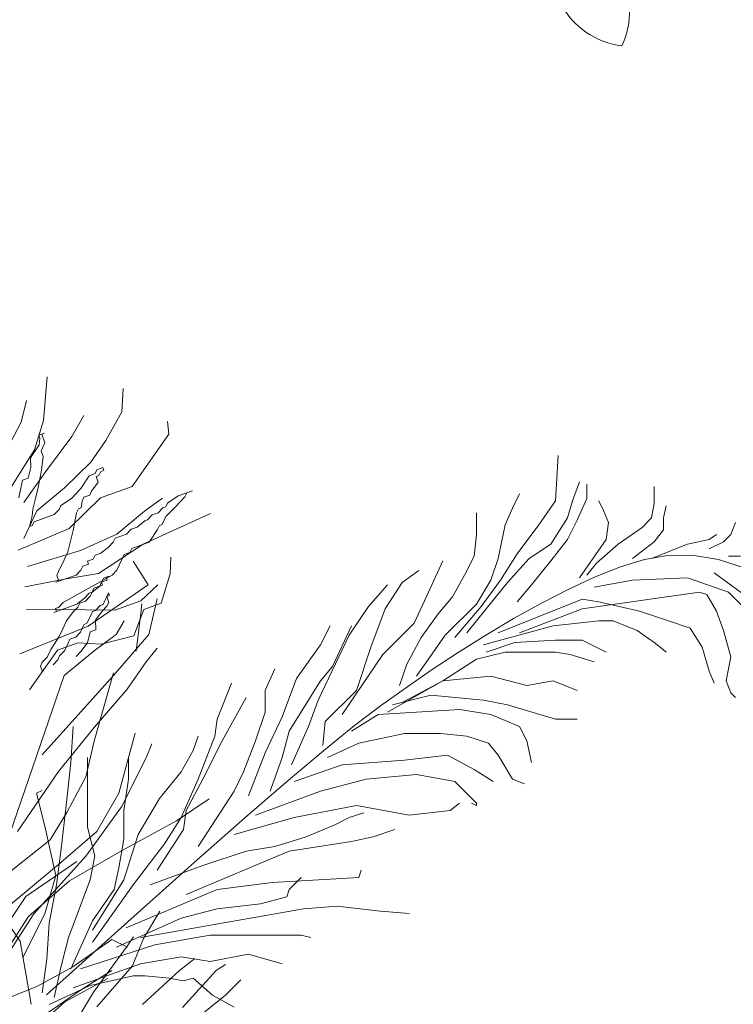
# Model space of a CAD drawing. Units: millimetres. Extents: x 595116 to 630915, y 909473 to 920225.
# Tile 74 of 134: x 629629.81 to 629636.468, y 919276.713 to 919285.898. Entities that reach past the tile are written whole.
import ezdxf

# ---------------------------------------------------------------- set-up
doc = ezdxf.new("R2010")
doc.units = ezdxf.units.MM
doc.layers.add('Dimension', color=3, linetype='Continuous', lineweight=18)
doc.layers.add('L-PLNT', color=85, linetype='Continuous', lineweight=13)
doc.styles.get("Standard").update_dxf_attribs({"font": 'arial.ttf'})
doc.dimstyles.new('ISO-25', dxfattribs={"dimtxt": 9, "dimasz": 6, "dimexe": 1.25, "dimexo": 0.625, "dimtad": 1, "dimlunit": 4, "dimtxsty": 'Standard', "dimcen": 2.5, "dimadec": 0, "dimazin": 0, "dimtfac": 1, "dimtmove": 0, "dimatfit": 3, "dimfxl": 1, "dimarcsym": 0})

# ---------------------------------------------------------------- blocks, each defined once
blk = doc.blocks.new('A$C4FB75ABC')
for p, q in [((2.8876, 3.7608), (2.897, 3.8696)), ((3.0823, 3.7823), (3.0858, 3.8403)), ((2.8322, 3.7571), (2.8454, 3.8105)), ((2.9584, 3.7215), (2.9885, 3.7729)), ((3.043, 3.7114), (3.0823, 3.7823)), ((2.7745, 3.6472), (2.8322, 3.7571)), ((2.8652, 3.6879), (2.8876, 3.7608)), ((3.1994, 3.7272), (3.1962, 3.7584)), ((2.8907, 3.7295), (2.8764, 3.7244)), ((2.8764, 3.7244), (2.8789, 3.7172)), ((2.8835, 3.727), (2.8907, 3.7295)), ((2.8913, 3.7054), (2.8835, 3.727)), ((2.893, 3.6331), (2.9584, 3.7215)), ((3.1085, 3.5972), (3.1994, 3.7272)), ((2.8769, 3.7003), (2.856, 3.6684)), ((2.8789, 3.7172), (2.8769, 3.7003)), ((2.8821, 3.6859), (2.8913, 3.7054)), ((3.0058, 3.6575), (3.043, 3.7114)), ((2.7932, 3.5729), (2.8652, 3.6879)), ((2.8873, 3.6716), (2.8821, 3.6859)), ((2.8833, 3.6377), (2.8873, 3.6716)), ((4.1608, 3.5609), (4.1668, 3.6742)), ((2.856, 3.6684), (2.8566, 3.6443)), ((2.9398, 3.5932), (3.0058, 3.6575)), ((2.8394, 3.5571), (2.893, 3.6331)), ((2.8566, 3.6443), (2.85, 3.6176)), ((2.8746, 3.5941), (2.8833, 3.6377)), ((3.0017, 3.6236), (2.9808, 3.5918)), ((3.0161, 3.6288), (3.0017, 3.6236)), ((3.0207, 3.6385), (3.0161, 3.6288)), ((3.0187, 3.6216), (3.0258, 3.6242)), ((3.035, 3.6437), (3.0207, 3.6385)), ((3.0258, 3.6242), (3.0304, 3.6339)), ((3.0304, 3.6339), (3.0376, 3.6365)), ((3.0376, 3.6365), (3.035, 3.6437)), ((2.8356, 3.6125), (2.827, 3.5688)), ((2.85, 3.6176), (2.8356, 3.6125)), ((3.0075, 3.5852), (3.0238, 3.6072)), ((3.0238, 3.6072), (3.0187, 3.6216)), ((4.2026, 3.5609), (4.2205, 3.6086)), ((4.2384, 3.5668), (4.2384, 3.6026)), ((2.868, 3.5674), (2.8746, 3.5941)), ((2.8712, 3.5361), (2.9398, 3.5932)), ((2.969, 3.5794), (2.9573, 3.5671)), ((2.9808, 3.5918), (2.969, 3.5794)), ((2.9885, 3.5702), (3.0029, 3.5754)), ((3.0029, 3.5754), (3.0075, 3.5852)), ((3.0296, 3.5688), (3.1085, 3.5972)), ((3.2224, 3.5733), (3.1962, 3.5558)), ((3.2582, 3.5862), (3.2224, 3.5733)), ((3.2393, 3.5713), (3.2439, 3.5811)), ((3.2439, 3.5811), (3.2582, 3.5862)), ((4.0535, 3.543), (4.0714, 3.5788)), ((4.4054, 3.5549), (4.4054, 3.5967)), ((2.8614, 3.5407), (2.868, 3.5674)), ((2.9312, 3.5496), (2.9266, 3.5398)), ((2.9573, 3.5671), (2.9312, 3.5496)), ((2.9518, 3.4922), (3.0296, 3.5688)), ((2.9819, 3.5435), (2.984, 3.5605)), ((2.984, 3.5605), (2.9885, 3.5702)), ((3.1389, 3.5352), (3.1839, 3.5676)), ((3.1962, 3.5558), (3.1917, 3.5461)), ((3.2158, 3.5466), (3.2393, 3.5713)), ((4.1191, 3.5013), (4.1608, 3.5609)), ((4.1907, 3.5192), (4.2026, 3.5609)), ((4.2145, 3.5132), (4.2384, 3.5668)), ((4.2801, 3.537), (4.2682, 3.5609)), ((4.3994, 3.5192), (4.4054, 3.5549)), ((4.4293, 3.5192), (4.4352, 3.549)), ((2.8391, 3.4678), (2.8712, 3.5361)), ((2.8594, 3.5238), (2.8614, 3.5407)), ((2.9148, 3.5275), (2.8646, 3.5094)), ((2.9266, 3.5398), (2.9148, 3.5275)), ((2.9616, 3.4876), (2.9702, 3.5312)), ((2.9702, 3.5312), (2.9748, 3.541)), ((2.9748, 3.541), (2.9819, 3.5435)), ((3.0703, 3.4781), (3.1389, 3.5352)), ((3.136, 3.4531), (3.303, 3.5294)), ((3.1584, 3.526), (3.1466, 3.5136)), ((3.1727, 3.5311), (3.1584, 3.526)), ((3.1845, 3.5435), (3.1727, 3.5311)), ((3.1917, 3.5461), (3.1845, 3.5435)), ((3.1922, 3.522), (3.2158, 3.5466)), ((3.964, 3.4774), (3.964, 3.5311)), ((4.0356, 3.5013), (4.0535, 3.543)), ((4.2921, 3.5072), (4.2801, 3.537)), ((2.8528, 3.4971), (2.8594, 3.5238)), ((2.8646, 3.5094), (2.86, 3.4997)), ((3.1394, 3.5111), (3.1205, 3.4961)), ((3.1466, 3.5136), (3.1394, 3.5111)), ((3.1713, 3.4901), (3.1759, 3.4999)), ((3.1759, 3.4999), (3.1831, 3.5024)), ((3.1831, 3.5024), (3.1922, 3.522)), ((4.0177, 3.4178), (4.0356, 3.5013)), ((4.0654, 3.4297), (4.1191, 3.5013)), ((4.1489, 3.4536), (4.1907, 3.5192)), ((4.1907, 3.4655), (4.2145, 3.5132)), ((4.2861, 3.4655), (4.2921, 3.5072)), ((4.3756, 3.4953), (4.3994, 3.5192)), ((4.4293, 3.4893), (4.4293, 3.5192)), ((4.5963, 3.4774), (4.6082, 3.5072)), ((2.8253, 3.4385), (2.9518, 3.4922)), ((2.86, 3.4997), (2.8528, 3.4971)), ((2.9484, 3.4342), (2.9616, 3.4876)), ((2.9797, 3.4374), (3.0703, 3.4781)), ((3.0944, 3.4786), (3.0657, 3.4683)), ((3.1062, 3.491), (3.0944, 3.4786)), ((3.1205, 3.4961), (3.1062, 3.491)), ((3.1503, 3.4583), (3.1713, 3.4901)), ((3.958, 3.4238), (3.964, 3.4774)), ((4.3159, 3.4536), (4.3756, 3.4953)), ((4.4054, 3.4595), (4.4293, 3.4893)), ((4.5426, 3.4655), (4.5605, 3.4774)), ((4.5784, 3.4595), (4.5963, 3.4774)), ((3.0244, 3.3805), (3.136, 3.4531)), ((3.0611, 3.4586), (3.0494, 3.4462)), ((3.0657, 3.4683), (3.0611, 3.4586)), ((3.1073, 3.4428), (3.1503, 3.4583)), ((4.0952, 3.4178), (4.1489, 3.4536)), ((4.1489, 3.4118), (4.1907, 3.4655)), ((4.2205, 3.3701), (4.2861, 3.4655)), ((4.2622, 3.4059), (4.3159, 3.4536)), ((4.3517, 3.4178), (4.4054, 3.4595)), ((4.3994, 3.4178), (4.4889, 3.4536)), ((4.4889, 3.4536), (4.5426, 3.4655)), ((4.5426, 3.4416), (4.5784, 3.4595)), ((2.848, 3.3981), (2.9797, 3.4374)), ((2.9392, 3.4147), (2.9484, 3.4342)), ((3.0304, 3.4313), (3.0161, 3.4262)), ((3.0494, 3.4462), (3.0304, 3.4313)), ((3.07, 3.3888), (3.0884, 3.4279)), ((3.0884, 3.4279), (3.1027, 3.433)), ((3.1027, 3.433), (3.1073, 3.4428)), ((4.0237, 3.3641), (4.0654, 3.4297)), ((2.9254, 3.3854), (2.9392, 3.4147)), ((2.9997, 3.4041), (2.9854, 3.3989)), ((3.0115, 3.4164), (2.9972, 3.4112)), ((2.9972, 3.4112), (2.9997, 3.4041)), ((3.0161, 3.4262), (3.0115, 3.4164)), ((3.1481, 3.3521), (3.1105, 3.4115)), ((3.2028, 3.3799), (3.2043, 3.4209)), ((3.8447, 3.3343), (3.8805, 3.4118)), ((3.9342, 3.3761), (3.958, 3.4238)), ((3.9998, 3.3641), (4.0177, 3.4178)), ((4.0415, 3.3582), (4.0952, 3.4178)), ((4.1012, 3.3522), (4.1489, 3.4118)), ((4.2384, 3.3761), (4.2622, 3.4059)), ((4.322, 3.3969), (4.3813, 3.4152)), ((4.3813, 3.4152), (4.4396, 3.4254)), ((4.4396, 3.4254), (4.5001, 3.426)), ((4.5001, 3.426), (4.5657, 3.4153)), ((4.5657, 3.4153), (4.6395, 3.3917)), ((4.5903, 3.4238), (4.6201, 3.4238)), ((2.9208, 3.3757), (2.9254, 3.3854)), ((2.9403, 3.3665), (3.0244, 3.3805)), ((2.9808, 3.3891), (2.969, 3.3768)), ((2.9854, 3.3989), (2.9808, 3.3891)), ((3.0583, 3.3765), (3.07, 3.3888)), ((3.1805, 3.307), (3.2028, 3.3799)), ((3.7791, 3.3582), (3.8208, 3.388)), ((4.2593, 3.3722), (4.322, 3.3969)), ((4.5545, 3.382), (4.6858, 3.2866)), ((2.8419, 3.3473), (2.9403, 3.3665)), ((2.969, 3.3768), (2.9188, 3.3587)), ((2.9188, 3.3587), (2.926, 3.3613)), ((2.926, 3.3613), (2.9208, 3.3757)), ((2.9369, 3.3085), (3.0583, 3.3765)), ((3.0322, 3.359), (3.0276, 3.3492)), ((3.0367, 3.3687), (3.0322, 3.359)), ((3.0322, 3.359), (3.0465, 3.3642)), ((3.0347, 3.3518), (3.0322, 3.359)), ((3.0511, 3.3739), (3.0367, 3.3687)), ((3.0439, 3.3713), (3.0511, 3.3739)), ((3.0465, 3.3642), (3.0439, 3.3713)), ((3.7373, 3.2926), (3.7791, 3.3582)), ((3.9044, 3.3224), (3.9342, 3.3761)), ((3.964, 3.3045), (3.9998, 3.3641)), ((3.9759, 3.2986), (4.0237, 3.3641)), ((3.9879, 3.2926), (4.0415, 3.3582)), ((4.1935, 3.342), (4.2593, 3.3722)), ((4.2563, 3.3463), (4.3517, 3.3641)), ((4.3517, 3.3641), (4.4889, 3.3701)), ((4.4889, 3.3701), (4.5903, 3.3343)), ((3.0015, 3.3317), (2.9897, 3.3194)), ((2.9986, 3.2497), (3.1481, 3.3521)), ((3.0086, 3.3343), (3.0015, 3.3317)), ((3.004, 3.3246), (3.0086, 3.3343)), ((3.0276, 3.3492), (3.0086, 3.3343)), ((3.0086, 3.3343), (3.0132, 3.3441)), ((3.0132, 3.3441), (3.0347, 3.3518)), ((3.0497, 3.3329), (3.0451, 3.3231)), ((3.0522, 3.3257), (3.0497, 3.3329)), ((3.1297, 3.313), (3.1722, 3.3526)), ((3.6956, 3.2986), (3.7433, 3.3522)), ((3.8089, 3.2568), (3.8447, 3.3343)), ((4.0654, 3.3105), (4.1012, 3.3522)), ((4.1256, 3.3072), (4.1935, 3.342)), ((4.2265, 3.2926), (4.5187, 3.3343)), ((4.5187, 3.3343), (4.5366, 3.3284)), ((4.5903, 3.3343), (4.644, 3.2807)), ((2.9708, 3.3045), (2.9134, 3.2838)), ((2.9251, 3.2962), (2.9369, 3.3085)), ((2.9897, 3.3194), (2.9708, 3.3045)), ((2.9733, 3.2973), (2.9779, 3.3071)), ((2.9779, 3.3071), (2.9923, 3.3122)), ((2.9923, 3.3122), (3.004, 3.3246)), ((3.0359, 3.3036), (3.0405, 3.3134)), ((3.0405, 3.3134), (3.0451, 3.3231)), ((3.0451, 3.3231), (3.0522, 3.3257)), ((3.0451, 3.3231), (3.0502, 3.3088)), ((3.0502, 3.3088), (3.0456, 3.299)), ((3.0651, 3.2898), (3.1297, 3.313)), ((3.1303, 3.2889), (3.1323, 3.3059)), ((3.1374, 3.2915), (3.1805, 3.307)), ((3.1501, 3.2292), (3.1706, 3.3178)), ((3.8686, 3.2807), (3.9044, 3.3224)), ((3.8865, 3.227), (3.964, 3.3045)), ((4.0177, 3.233), (4.2265, 3.3164)), ((4.0565, 3.2687), (4.1256, 3.3072)), ((4.2265, 3.3164), (4.2682, 3.3105)), ((4.2682, 3.3105), (4.3696, 3.2866)), ((4.5366, 3.3284), (4.5605, 3.2866)), ((2.8457, 3.2919), (3.0651, 3.2898)), ((2.9134, 3.2838), (2.9206, 3.2864)), ((2.918, 3.2936), (2.9251, 3.2962)), ((2.9206, 3.2864), (2.918, 3.2936)), ((2.9452, 3.2629), (2.9616, 3.285)), ((2.9616, 3.285), (2.9733, 3.2973)), ((3.0052, 3.2763), (3.0098, 3.2861)), ((3.0098, 3.2861), (3.0169, 3.2887)), ((3.0169, 3.2887), (3.0287, 3.301)), ((3.0339, 3.2867), (3.0175, 3.2646)), ((3.0287, 3.301), (3.0359, 3.3036)), ((3.0456, 3.299), (3.0339, 3.2867)), ((3.1125, 3.2258), (3.1374, 3.2915)), ((3.1182, 3.1873), (3.1303, 3.2889)), ((3.6479, 3.227), (3.6956, 3.2986)), ((3.7015, 3.1972), (3.7373, 3.2926)), ((3.8268, 3.2211), (3.8686, 3.2807)), ((3.9103, 3.2211), (3.9759, 3.2986)), ((3.9401, 3.233), (3.9879, 3.2926)), ((4.0714, 3.233), (4.2265, 3.2926)), ((4.3696, 3.2866), (4.4412, 3.2628)), ((4.5605, 3.2866), (4.5784, 3.2389)), ((2.936, 3.2434), (2.9452, 3.2629)), ((2.9888, 3.2542), (2.996, 3.2568)), ((2.996, 3.2568), (3.0052, 3.2763)), ((3.0175, 3.2646), (3.0181, 3.2405)), ((3.0684, 3.2292), (3.0888, 3.2633)), ((3.7314, 3.1793), (3.8089, 3.2568)), ((3.9871, 3.2274), (4.0565, 3.2687)), ((4.1549, 3.2509), (4.2682, 3.2628)), ((4.2682, 3.2628), (4.304, 3.2628)), ((4.304, 3.2628), (4.3637, 3.2389)), ((4.4412, 3.2628), (4.4949, 3.2449)), ((2.829, 3.1805), (2.9986, 3.2497)), ((2.9269, 3.2238), (2.936, 3.2434)), ((2.9679, 3.2224), (2.9797, 3.2347)), ((2.9797, 3.2347), (2.9842, 3.2445)), ((2.9842, 3.2445), (2.9888, 3.2542)), ((3.0038, 3.2353), (2.9972, 3.2086)), ((3.0181, 3.2405), (3.0038, 3.2353)), ((3.5763, 3.2032), (3.6001, 3.2509)), ((3.6061, 3.1495), (3.6538, 3.2509)), ((3.9819, 3.2032), (4.1549, 3.2509)), ((4.3637, 3.2389), (4.4054, 3.2091)), ((4.4949, 3.2449), (4.5247, 3.1972)), ((4.5784, 3.2389), (4.5963, 3.1734)), ((2.9059, 3.192), (2.9269, 3.2238)), ((2.9229, 3.19), (2.9731, 3.208)), ((2.9398, 3.188), (2.949, 3.2075)), ((2.949, 3.2075), (2.9535, 3.2172)), ((2.9535, 3.2172), (2.9679, 3.2224)), ((2.9731, 3.208), (3.031, 3.2046)), ((2.9972, 3.2086), (2.9808, 3.1865)), ((3.0139, 3.1884), (3.0684, 3.2292)), ((3.031, 3.2046), (3.1125, 3.2258)), ((3.0616, 3.1271), (3.1501, 3.2292)), ((3.5703, 3.066), (3.6479, 3.227)), ((3.791, 3.1555), (3.8268, 3.2211)), ((3.8149, 3.1257), (3.8865, 3.227)), ((3.9185, 3.1843), (3.9871, 3.2274)), ((3.9879, 3.1853), (4.0594, 3.2091)), ((4.0594, 3.2091), (4.1608, 3.2151)), ((4.1608, 3.2151), (4.2265, 3.2151)), ((4.2265, 3.2151), (4.2861, 3.1853)), ((4.4054, 3.2091), (4.4293, 3.1912)), ((2.8529, 3.0918), (2.9229, 3.19)), ((2.8967, 3.1725), (2.9059, 3.192)), ((2.928, 3.1756), (2.9398, 3.188)), ((2.9389, 3.1271), (3.0139, 3.1884)), ((2.9808, 3.1865), (2.969, 3.1742)), ((3.1433, 3.1611), (3.1706, 3.1952)), ((3.5166, 3.1197), (3.5763, 3.2032)), ((3.6658, 3.0899), (3.7015, 3.1972)), ((3.8516, 3.1401), (3.9185, 3.1843)), ((3.964, 3.1674), (4.0356, 3.1853)), ((4.0356, 3.1853), (4.1072, 3.1853)), ((4.1072, 3.1853), (4.1608, 3.1853)), ((4.1608, 3.1853), (4.1966, 3.1793)), ((4.4293, 3.1912), (4.4352, 3.1853)), ((4.5247, 3.1972), (4.5426, 3.1376)), ((2.8804, 3.1504), (2.885, 3.1601)), ((2.885, 3.1601), (2.8967, 3.1725)), ((2.9117, 3.1535), (2.9234, 3.1659)), ((2.9234, 3.1659), (2.928, 3.1756)), ((3.0956, 3.093), (3.1433, 3.1611)), ((3.63, 3.0303), (3.7314, 3.1793)), ((3.8805, 3.1137), (3.964, 3.1674)), ((4.1966, 3.1793), (4.2563, 3.1614)), ((4.5963, 3.1734), (4.5844, 3.1137)), ((2.8856, 3.136), (2.8804, 3.1504)), ((3.0139, 2.9637), (3.0616, 3.1339)), ((3.4391, 3.0899), (3.4629, 3.1436)), ((3.5763, 3.1137), (3.6061, 3.1495)), ((3.7731, 3.1018), (3.791, 3.1555)), ((3.7873, 3.0958), (3.8516, 3.1401)), ((4.5426, 3.1376), (4.5545, 3.1078)), ((2.7823, 2.6709), (2.9389, 3.1271)), ((2.8844, 2.9296), (3.0616, 3.1271)), ((3.4808, 3.0243), (3.5166, 3.1197)), ((3.4987, 2.9885), (3.5763, 3.1137)), ((3.7433, 3.0362), (3.8805, 3.1137)), ((3.7791, 3.0601), (3.8805, 3.1137)), ((3.8805, 3.1137), (3.9998, 3.1257)), ((3.9998, 3.1257), (4.0893, 3.1018)), ((4.0893, 3.1018), (4.1549, 3.1137)), ((4.1549, 3.1137), (4.2145, 3.0899)), ((4.5844, 3.1137), (4.5963, 3.0839)), ((3.0139, 2.9977), (3.0956, 3.093)), ((3.3198, 3.0184), (3.3556, 3.1078)), ((3.4391, 3.0362), (3.4391, 3.0899)), ((3.5882, 3.0124), (3.6658, 3.0899)), ((3.7254, 3.0513), (3.7873, 3.0958)), ((4.5963, 3.0839), (4.6082, 3.072)), ((3.3317, 2.9647), (3.3914, 3.072)), ((3.5465, 3.0005), (3.5703, 3.066)), ((3.7552, 3.0541), (3.8507, 3.078)), ((3.8507, 3.078), (3.9819, 3.066)), ((3.9819, 3.066), (4.0415, 3.0541)), ((3.4152, 2.9647), (3.4391, 3.0362)), ((3.6611, 3.0024), (3.7254, 3.0513)), ((3.7194, 3.0303), (3.8149, 3.0362)), ((3.8149, 3.0362), (3.9222, 3.0422)), ((3.9222, 3.0422), (3.9998, 3.0303)), ((4.0415, 3.0541), (4.1608, 3.0184)), ((3.3138, 2.9766), (3.3198, 3.0184)), ((3.4391, 2.9349), (3.4808, 3.0243)), ((3.5822, 2.9528), (3.5882, 3.0124)), ((3.6538, 2.9885), (3.7194, 3.0303)), ((3.9998, 3.0303), (4.0714, 3.0005)), ((4.1608, 3.0184), (4.2145, 3.0184)), ((2.9253, 2.8888), (3.0139, 2.9977)), ((2.9559, 2.911), (2.9619, 3.0005)), ((3.4808, 2.923), (3.4987, 2.9885)), ((3.5047, 2.9051), (3.5465, 3.0005)), ((3.5886, 2.9442), (3.6611, 3.0024)), ((4.0714, 3.0005), (4.0893, 2.9647)), ((2.9935, 2.8751), (3.0139, 2.9637)), ((3.0752, 2.8343), (3.1161, 2.9841)), ((3.2601, 2.9408), (3.2721, 2.9766)), ((3.2721, 2.8693), (3.3138, 2.9766)), ((3.284, 2.8693), (3.3317, 2.9647)), ((3.3854, 2.8872), (3.4152, 2.9647)), ((3.6717, 2.9587), (3.7851, 2.9826)), ((3.7851, 2.9826), (3.8745, 2.9826)), ((3.8745, 2.9826), (3.9401, 2.9766)), ((3.9401, 2.9766), (3.9938, 2.9587)), ((4.0893, 2.9647), (4.1012, 2.911)), ((3.1433, 2.9228), (3.157, 2.9569)), ((3.2303, 2.8872), (3.2601, 2.9408)), ((3.5019, 2.8714), (3.5886, 2.9442)), ((3.5942, 2.923), (3.6717, 2.9587)), ((3.9938, 2.9587), (4.0177, 2.9289)), ((2.9977, 2.8216), (2.9977, 2.923)), ((3.082, 2.8002), (3.1433, 2.9228)), ((3.0991, 2.8693), (3.0991, 2.923)), ((3.3973, 2.8276), (3.4391, 2.9349)), ((3.451, 2.8395), (3.4808, 2.923)), ((3.63, 2.9051), (3.7851, 2.917)), ((3.7851, 2.917), (3.8924, 2.9289)), ((3.8924, 2.9289), (3.958, 2.8932)), ((4.0177, 2.9289), (4.0535, 2.8693)), ((2.8231, 2.739), (2.9253, 2.8888)), ((2.944, 2.8037), (2.9559, 2.911)), ((3.5107, 2.8633), (3.63, 2.9051)), ((3.958, 2.8932), (4.0058, 2.8633)), ((2.9458, 2.7866), (2.9935, 2.8751)), ((3.0872, 2.7918), (3.0991, 2.8693)), ((3.1766, 2.8216), (3.2303, 2.8872)), ((3.2303, 2.7739), (3.2721, 2.8693)), ((3.2422, 2.7918), (3.284, 2.8693)), ((3.3615, 2.8395), (3.3854, 2.8872)), ((3.3951, 2.779), (3.5019, 2.8714)), ((3.5763, 2.8395), (3.6896, 2.8693)), ((3.6896, 2.8693), (3.8149, 2.8812)), ((3.8149, 2.8812), (3.9103, 2.8633)), ((4.0535, 2.8693), (4.0833, 2.8574)), ((2.8708, 2.8343), (2.8844, 2.8411)), ((3.2721, 2.7024), (3.3615, 2.8395)), ((3.4152, 2.7799), (3.5763, 2.8395)), ((3.9103, 2.8633), (3.964, 2.8097)), ((2.8913, 2.7526), (2.8708, 2.8343)), ((2.9977, 2.7501), (2.9977, 2.8216)), ((3.0207, 2.739), (3.0752, 2.8343)), ((3.1229, 2.7322), (3.1766, 2.8216)), ((3.2183, 2.7662), (3.3, 2.8207)), ((2.9321, 2.6964), (2.944, 2.8037)), ((2.9935, 2.6777), (3.082, 2.8002)), ((3.0872, 2.7203), (3.0872, 2.7918)), ((3.2363, 2.7441), (3.2422, 2.7918)), ((3.5107, 2.7739), (3.6658, 2.8037)), ((3.6658, 2.8037), (3.797, 2.7799)), ((3.797, 2.7799), (3.8984, 2.7918)), ((3.8984, 2.7918), (3.9222, 2.8097)), ((3.964, 2.8037), (3.9521, 2.8097)), ((3.964, 2.8097), (3.964, 2.8037)), ((2.9049, 2.7185), (2.9458, 2.7866)), ((3.082, 2.6913), (3.2183, 2.7662)), ((3.1886, 2.7083), (3.2303, 2.7739)), ((3.2623, 2.6619), (3.3951, 2.779)), ((3.3615, 2.7322), (3.5107, 2.7739)), ((3.6121, 2.756), (3.6479, 2.7739)), ((3.6479, 2.7739), (3.6837, 2.7858)), ((2.9185, 2.63), (2.8913, 2.7526)), ((3.0156, 2.6785), (2.9977, 2.7501)), ((3.1707, 2.6428), (3.2363, 2.7441)), ((3.5405, 2.7262), (3.6121, 2.756)), ((3.7075, 2.7262), (3.7612, 2.7441)), ((2.7414, 2.5891), (2.9049, 2.7185)), ((2.9253, 2.6572), (3.0207, 2.739)), ((3.0752, 2.6487), (3.0872, 2.7203)), ((3.0872, 2.6189), (3.1229, 2.7322)), ((3.4629, 2.7024), (3.5405, 2.7262)), ((3.6538, 2.7143), (3.7075, 2.7262)), ((2.9201, 2.607), (2.9321, 2.6964)), ((3.111, 2.607), (3.1886, 2.7083)), ((3.3914, 2.6904), (3.4629, 2.7024)), ((3.4987, 2.6904), (3.6538, 2.7143)), ((2.864, 2.5347), (2.9935, 2.6777)), ((2.9526, 2.6164), (3.082, 2.6913)), ((3.0036, 2.6189), (3.0156, 2.6785)), ((3.2422, 2.5831), (3.4987, 2.6904)), ((3.284, 2.6547), (3.3914, 2.6904)), ((2.7209, 2.487), (2.9253, 2.6572)), ((2.8442, 2.5778), (2.9704, 2.6651)), ((3.0633, 2.5951), (3.0752, 2.6487)), ((3.0976, 2.5149), (3.2623, 2.6619)), ((3.1528, 2.607), (3.284, 2.6547)), ((2.8913, 2.5347), (2.9185, 2.63)), ((2.95, 2.4758), (3.0036, 2.6189)), ((3.0096, 2.4937), (3.0872, 2.6189)), ((3.457, 2.6129), (3.6717, 2.6249)), ((3.4987, 2.5951), (3.5286, 2.6249)), ((3.6717, 2.6249), (3.6777, 2.6428)), ((2.8504, 2.5279), (2.9526, 2.6164)), ((2.9022, 2.5116), (2.9201, 2.607)), ((3.0096, 2.4639), (3.111, 2.607)), ((3.0096, 2.5176), (3.0633, 2.5951)), ((3.0931, 2.4997), (3.3198, 2.5951)), ((3.3198, 2.5951), (3.457, 2.6129)), ((3.4928, 2.5772), (3.4987, 2.5951)), ((2.786, 2.4905), (2.8442, 2.5778)), ((3.4272, 2.5593), (3.4928, 2.5772)), ((2.8299, 2.4666), (2.7686, 2.5551)), ((3.1289, 2.4758), (3.5345, 2.5474)), ((3.2303, 2.5235), (3.3198, 2.5474)), ((3.3198, 2.5474), (3.4272, 2.5593)), ((3.5345, 2.5474), (3.618, 2.5533)), ((3.618, 2.5533), (3.7254, 2.5414)), ((2.7891, 2.4325), (2.8504, 2.5279)), ((2.8027, 2.4393), (2.864, 2.5347)), ((2.8368, 2.4257), (2.8913, 2.5347)), ((3.0693, 2.452), (3.2303, 2.5235)), ((3.1365, 2.4734), (3.1774, 2.5415)), ((3.7254, 2.5414), (3.797, 2.5354)), ((2.895, 2.333), (3.0976, 2.5149)), ((2.8963, 2.4222), (2.9022, 2.5116)), ((2.9559, 2.3983), (3.0096, 2.5176)), ((2.9321, 2.4043), (2.95, 2.4758)), ((3.0962, 2.4544), (3.1115, 2.4773)), ((3.1093, 2.4053), (3.1365, 2.4734)), ((3.1647, 2.4579), (3.3019, 2.4818)), ((3.3019, 2.4818), (3.4152, 2.4818)), ((3.4152, 2.4818), (3.5286, 2.4818)), ((3.5286, 2.4818), (3.5524, 2.4758)), ((2.8572, 2.31), (2.8299, 2.4666)), ((2.9607, 2.4032), (3.0578, 2.4711)), ((2.9798, 2.3983), (3.1647, 2.4579)), ((3.0123, 2.3401), (3.0962, 2.4544)), ((3.0578, 2.4711), (3.0966, 2.4517)), ((3.1289, 2.4102), (3.2303, 2.4281)), ((3.2259, 2.3934), (3.264, 2.4239)), ((3.2303, 2.4281), (3.3019, 2.4162)), ((3.3019, 2.4162), (3.3973, 2.4341)), ((3.3973, 2.4341), (3.4808, 2.4102)), ((2.8733, 2.3546), (2.9607, 2.4032)), ((2.8844, 2.3387), (2.8963, 2.4222)), ((2.9142, 2.3268), (2.9321, 2.4043)), ((2.9619, 2.3506), (3.1289, 2.4102)), ((3.0207, 2.3031), (3.1093, 2.4053)), ((3.3174, 2.3934), (3.3403, 2.4087)), ((2.9413, 2.3158), (3.0481, 2.3741)), ((2.9801, 2.3449), (3.0578, 2.3935)), ((3.0036, 2.3566), (3.111, 2.3804)), ((3.111, 2.3804), (3.1408, 2.3804)), ((3.1344, 2.3096), (3.2259, 2.3934)), ((3.1408, 2.3804), (3.2005, 2.3745)), ((3.2005, 2.3745), (3.2363, 2.3685)), ((3.2335, 2.302), (3.3174, 2.3934)), ((3.2363, 2.3685), (3.2601, 2.3745)), ((3.2601, 2.3745), (3.3079, 2.3327)), ((2.7277, 2.2964), (2.8733, 2.3546)), ((2.9022, 2.3089), (3.0036, 2.3566)), ((3.3403, 2.3324), (3.3784, 2.3706)), ((2.8539, 2.2576), (2.9801, 2.3449)), ((2.9666, 2.2638), (3.0123, 2.3401)), ((3.264, 2.2715), (3.3403, 2.3324)), ((3.3079, 2.3327), (3.3615, 2.3029)), ((2.8539, 2.2382), (2.9413, 2.3158))]:
    blk.add_line(p, q)
blk = doc.blocks.new('A$C77972600')
for centre, radius, start, end in [((2.0484, 1.3855), 0.2106, 152.1384, 263.3149), ((1.8257, 1.2684), 0.2185, 335.0581, 80.3951)]:
    blk.add_arc(centre, radius, start, end)
blk = doc.blocks.new('*D216')
at = {"layer": 'Defpoints', "color": 0, "transparency": 16777216}
for p in [(629743.5408, 919411.9276), (629505.0408, 919411.8279), (629743.5408, 918832.3776)]:
    blk.add_point(p, dxfattribs=at)
at = {"layer": 'Dimension', "color": 0, "lineweight": -2, "transparency": 16777216}
for p, q in [((629743.5408, 919411.3026), (629743.5408, 918831.1276)), ((629505.0408, 919411.2029), (629505.0408, 918831.1276)), ((629511.0408, 918832.3776), (629737.5408, 918832.3776))]:
    blk.add_line(p, q, dxfattribs=at)
at = {"layer": 'Dimension', "color": 0, "transparency": 16777216}
for points in [[(629511.0408, 918833.3776), (629511.0408, 918831.3776), (629505.0408, 918832.3776)], [(629737.5408, 918833.3776), (629737.5408, 918831.3776), (629743.5408, 918832.3776)]]:
    blk.add_solid(points, dxfattribs=at)
at = {"layer": 'Dimension', "color": 0, "transparency": 16777216, "insert": (629624.2908, 918837.656), "char_height": 9, "attachment_point": 5}
blk.add_mtext('19\'-10 1/2"', dxfattribs=at)

msp = doc.modelspace()

# ---------------------------------------------------------------- block references
at = {"layer": 'L-PLNT'}
for name, p, xscale, yscale, zscale in [('A$C77972600', (629628.3195, 919281.5233), 3.512546757812034, 3.512546757812034, 3.512546757812034), ('A$C4FB75ABC', (629619.1929, 919268.043), 3.753413438031968, 3.753413438031968, 3.753413438031968)]:
    msp.add_blockref(name, p, dxfattribs=dict(at, xscale=xscale, yscale=yscale, zscale=zscale))

# ---------------------------------------------------------------- dimensions: what is measured, and where the dimension line sits
at = {"layer": 'Dimension'}
dim = msp.add_linear_dim(base=(629743.5408, 918832.3776), p1=(629505.0408, 919411.8279), p2=(629743.5408, 919411.9276), dimstyle='ISO-25', override={"dimdec": 1, "dimlfac": 1, "dimrnd": 0, "dimzin": 1, "dimdsep": 46, "dimlunit": 4, "dimfrac": 2}, dxfattribs=at)
dim.commit()
dim.dimension.update_dxf_attribs({"geometry": '*D216', "text_midpoint": (629624.2908, 918837.656)})

doc.saveas('drawing.dxf')
